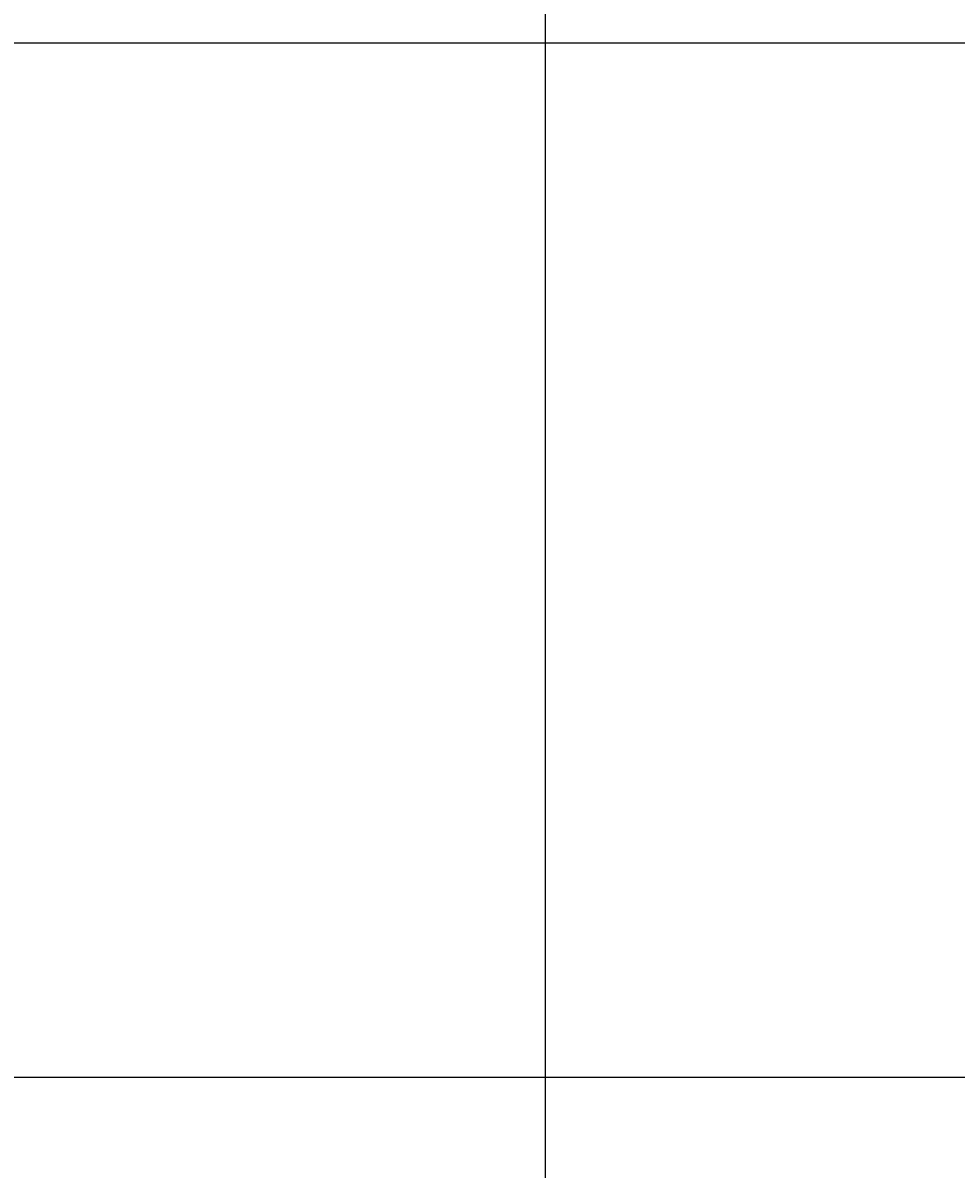
# Model space of a CAD drawing. Units: inches. Extents: x 35362 to 73946, y 43607 to 67532.
# Tile 18 of 134: x 47763 to 48148, y 46091 to 46564. Entities that reach past the tile are written whole.
import ezdxf

# ---------------------------------------------------------------- set-up
doc = ezdxf.new("R2010")
doc.units = ezdxf.units.IN
doc.header["$MEASUREMENT"] = 0
doc.layers.add('A-ANNO-DIMS', color=2, linetype='Continuous', lineweight=18)
doc.styles.get("Standard").update_dxf_attribs({"font": 'arial.ttf'})
doc.dimstyles.get("Standard").update_dxf_attribs({"dimtxt": 0.18, "dimasz": 0.18, "dimexe": 0.18, "dimexo": 0.0625, "dimgap": 0.09, "dimtad": 0, "dimtih": 1, "dimtoh": 1, "dimdec": 4, "dimzin": 0, "dimdsep": 46, "dimtxsty": 'Standard', "dimcen": 0.09, "dimadec": 0, "dimazin": 0, "dimtfac": 1, "dimtdec": 4, "dimtofl": 0, "dimtmove": 0, "dimatfit": 3, "dimfxl": 1, "dimtolj": 1, "dimtzin": 0, "dimarcsym": 0})

# ---------------------------------------------------------------- blocks, each defined once
blk = doc.blocks.new('*D5')
at = {"layer": 'A-ANNO-DIMS', "color": 0, "lineweight": -2, "transparency": 16777216}
for p, q in [((37121.95, 46919.32), (37121.95, 43606.68)), ((69871.5, 45449.83), (69871.5, 43606.68)), ((37122.13, 43606.86), (53496.29, 43606.86)), ((69871.32, 43606.86), (53497.15, 43606.86))]:
    blk.add_line(p, q, dxfattribs=at)
at = {"layer": 'A-ANNO-DIMS', "color": 0, "transparency": 16777216}
for points in [[(37122.13, 43606.89), (37122.13, 43606.83), (37121.95, 43606.86)], [(69871.32, 43606.89), (69871.32, 43606.83), (69871.5, 43606.86)]]:
    blk.add_solid(points, dxfattribs=at)
at = {"layer": 'Defpoints', "color": 0, "transparency": 16777216}
for p in [(37121.95, 46919.38), (69871.5, 45449.89), (69871.5, 43606.86)]:
    blk.add_point(p, dxfattribs=at)
at = {"layer": 'A-ANNO-DIMS', "color": 0, "transparency": 16777216, "insert": (53496.72, 43606.86), "char_height": 0.18, "attachment_point": 5}
blk.add_mtext('\\A1;32750', dxfattribs=at)
blk = doc.blocks.new('*D11')
at = {"layer": 'A-ANNO-DIMS', "color": 0, "lineweight": -2, "transparency": 16777216}
for p, q in [((47978.66, 56028.77), (47978.66, 43606.68)), ((53109.76, 56028.77), (53109.76, 43606.68)), ((47978.84, 43606.86), (50543.87, 43606.86)), ((53109.58, 43606.86), (50544.55, 43606.86))]:
    blk.add_line(p, q, dxfattribs=at)
at = {"layer": 'A-ANNO-DIMS', "color": 0, "transparency": 16777216}
for points in [[(47978.84, 43606.89), (47978.84, 43606.83), (47978.66, 43606.86)], [(53109.58, 43606.89), (53109.58, 43606.83), (53109.76, 43606.86)]]:
    blk.add_solid(points, dxfattribs=at)
at = {"layer": 'Defpoints', "color": 0, "transparency": 16777216}
for p in [(47978.66, 56028.84), (53109.76, 56028.84), (53109.76, 43606.86)]:
    blk.add_point(p, dxfattribs=at)
at = {"layer": 'A-ANNO-DIMS', "color": 0, "transparency": 16777216, "insert": (50544.21, 43606.86), "char_height": 0.18, "attachment_point": 5}
blk.add_mtext('\\A1;5131', dxfattribs=at)
blk = doc.blocks.new('*D27')
at = {"layer": 'A-ANNO-DIMS', "color": 0, "lineweight": -2, "transparency": 16777216}
for p, q in [((47978.66, 56028.77), (47978.66, 43606.68)), ((48373.49, 53428.96), (48373.49, 43606.68)), ((47978.84, 43606.86), (48175.68, 43606.86)), ((48373.31, 43606.86), (48176.47, 43606.86))]:
    blk.add_line(p, q, dxfattribs=at)
at = {"layer": 'A-ANNO-DIMS', "color": 0, "transparency": 16777216}
for points in [[(47978.84, 43606.89), (47978.84, 43606.83), (47978.66, 43606.86)], [(48373.31, 43606.89), (48373.31, 43606.83), (48373.49, 43606.86)]]:
    blk.add_solid(points, dxfattribs=at)
at = {"layer": 'Defpoints', "color": 0, "transparency": 16777216}
for p in [(47978.66, 56028.84), (48373.49, 53429.02), (48373.49, 43606.86)]:
    blk.add_point(p, dxfattribs=at)
at = {"layer": 'A-ANNO-DIMS', "color": 0, "transparency": 16777216, "insert": (48176.08, 43606.86), "char_height": 0.18, "attachment_point": 5}
blk.add_mtext('\\A1;394.8', dxfattribs=at)
blk = doc.blocks.new('*D67')
at = {"layer": 'A-ANNO-DIMS', "color": 0, "lineweight": -2, "transparency": 16777216}
for p, q in [((56873.54, 53351.53), (35361.77, 53351.53)), ((35361.95, 53351.35), (35361.95, 49400.89)), ((35361.95, 45450.07), (35361.95, 49400.53)), ((53793.58, 45449.89), (35361.77, 45449.89))]:
    blk.add_line(p, q, dxfattribs=at)
at = {"layer": 'A-ANNO-DIMS', "color": 0, "transparency": 16777216}
for points in [[(35361.92, 53351.35), (35361.98, 53351.35), (35361.95, 53351.53)], [(35361.92, 45450.07), (35361.98, 45450.07), (35361.95, 45449.89)]]:
    blk.add_solid(points, dxfattribs=at)
at = {"layer": 'Defpoints', "color": 0, "transparency": 16777216}
for p in [(35361.95, 53351.53), (56873.6, 53351.53), (53793.64, 45449.89)]:
    blk.add_point(p, dxfattribs=at)
at = {"layer": 'A-ANNO-DIMS', "color": 0, "transparency": 16777216, "insert": (35361.95, 49400.71), "char_height": 0.18, "attachment_point": 5}
blk.add_mtext('\\A1;7901.6', dxfattribs=at)
blk = doc.blocks.new('*D76')
at = {"layer": 'A-ANNO-DIMS', "color": 0, "lineweight": -2, "transparency": 16777216}
for p, q in [((54052.84, 46555.29), (35361.77, 46555.29)), ((35361.95, 46555.11), (35361.95, 46342.27)), ((35361.95, 46129.06), (35361.95, 46341.9)), ((53793.58, 46128.88), (35361.77, 46128.88))]:
    blk.add_line(p, q, dxfattribs=at)
at = {"layer": 'A-ANNO-DIMS', "color": 0, "transparency": 16777216}
for points in [[(35361.92, 46555.11), (35361.98, 46555.11), (35361.95, 46555.29)], [(35361.92, 46129.06), (35361.98, 46129.06), (35361.95, 46128.88)]]:
    blk.add_solid(points, dxfattribs=at)
at = {"layer": 'Defpoints', "color": 0, "transparency": 16777216}
for p in [(35361.95, 46555.29), (54052.9, 46555.29), (53793.64, 46128.88)]:
    blk.add_point(p, dxfattribs=at)
at = {"layer": 'A-ANNO-DIMS', "color": 0, "transparency": 16777216, "insert": (35361.95, 46342.09), "char_height": 0.18, "attachment_point": 5}
blk.add_mtext('\\A1;426.4', dxfattribs=at)
blk = doc.blocks.new('*D90')
at = {"layer": 'A-ANNO-DIMS', "color": 0, "lineweight": -2, "transparency": 16777216}
for p, q in [((53707.72, 47291.29), (35361.77, 47291.29)), ((35361.95, 47291.11), (35361.95, 46710.26)), ((35361.95, 46129.06), (35361.95, 46709.9)), ((53793.58, 46128.88), (35361.77, 46128.88))]:
    blk.add_line(p, q, dxfattribs=at)
at = {"layer": 'A-ANNO-DIMS', "color": 0, "transparency": 16777216}
for points in [[(35361.92, 47291.11), (35361.98, 47291.11), (35361.95, 47291.29)], [(35361.92, 46129.06), (35361.98, 46129.06), (35361.95, 46128.88)]]:
    blk.add_solid(points, dxfattribs=at)
at = {"layer": 'Defpoints', "color": 0, "transparency": 16777216}
for p in [(53707.78, 47291.29), (35361.95, 46128.88), (53793.64, 46128.88)]:
    blk.add_point(p, dxfattribs=at)
at = {"layer": 'A-ANNO-DIMS', "color": 0, "transparency": 16777216, "insert": (35361.95, 46710.08), "char_height": 0.18, "attachment_point": 5}
blk.add_mtext('\\A1;1162.4', dxfattribs=at)

msp = doc.modelspace()

# ---------------------------------------------------------------- dimensions: what is measured, and where the dimension line sits
at = {"layer": 'A-ANNO-DIMS'}
for base, p1, p2, override, picture, middle in [((53109.76, 43606.859), (47978.665, 56028.836), (53109.76, 56028.836), {"dimdec": 0, "dimlfac": 1, "dimrnd": 0, "dimzin": 0, "dimdsep": 46, "dimlunit": 2}, '*D11', (50544.212, 43606.859)), ((48373.492, 43606.859), (47978.665, 56028.836), (48373.492, 53429.019), {"dimdec": 1, "dimlfac": 1, "dimrnd": 0, "dimzin": 0, "dimdsep": 46, "dimlunit": 2}, '*D27', (48176.078, 43606.859)), ((69871.496, 43606.859), (37121.949, 46919.381), (69871.496, 45449.894), {"dimdec": 0, "dimlfac": 1, "dimrnd": 0, "dimzin": 0, "dimdsep": 46, "dimlunit": 2}, '*D5', (53496.723, 43606.859))]:
    dim = msp.add_linear_dim(base=base, p1=p1, p2=p2, dimstyle='Standard', override=override, dxfattribs=at)
    dim.commit()
    dim.dimension.update_dxf_attribs({"geometry": picture, "text_midpoint": middle})
for base, p1, p2, picture, middle in [((35361.949, 53351.529), (53793.638, 45449.894), (56873.602, 53351.529), '*D67', (35361.949, 49400.712)), ((35361.949, 46128.878), (53707.781, 47291.285), (53793.638, 46128.878), '*D90', (35361.949, 46710.081)), ((35361.949, 46555.293), (53793.638, 46128.878), (54052.899, 46555.293), '*D76', (35361.949, 46342.086))]:
    dim = msp.add_linear_dim(base=base, p1=p1, p2=p2, angle=90, dimstyle='Standard', override={"dimdec": 1, "dimlfac": 1, "dimrnd": 0, "dimzin": 0, "dimdsep": 46, "dimlunit": 2}, dxfattribs=at)
    dim.commit()
    dim.dimension.update_dxf_attribs({"geometry": picture, "text_midpoint": middle})

doc.saveas('drawing.dxf')
